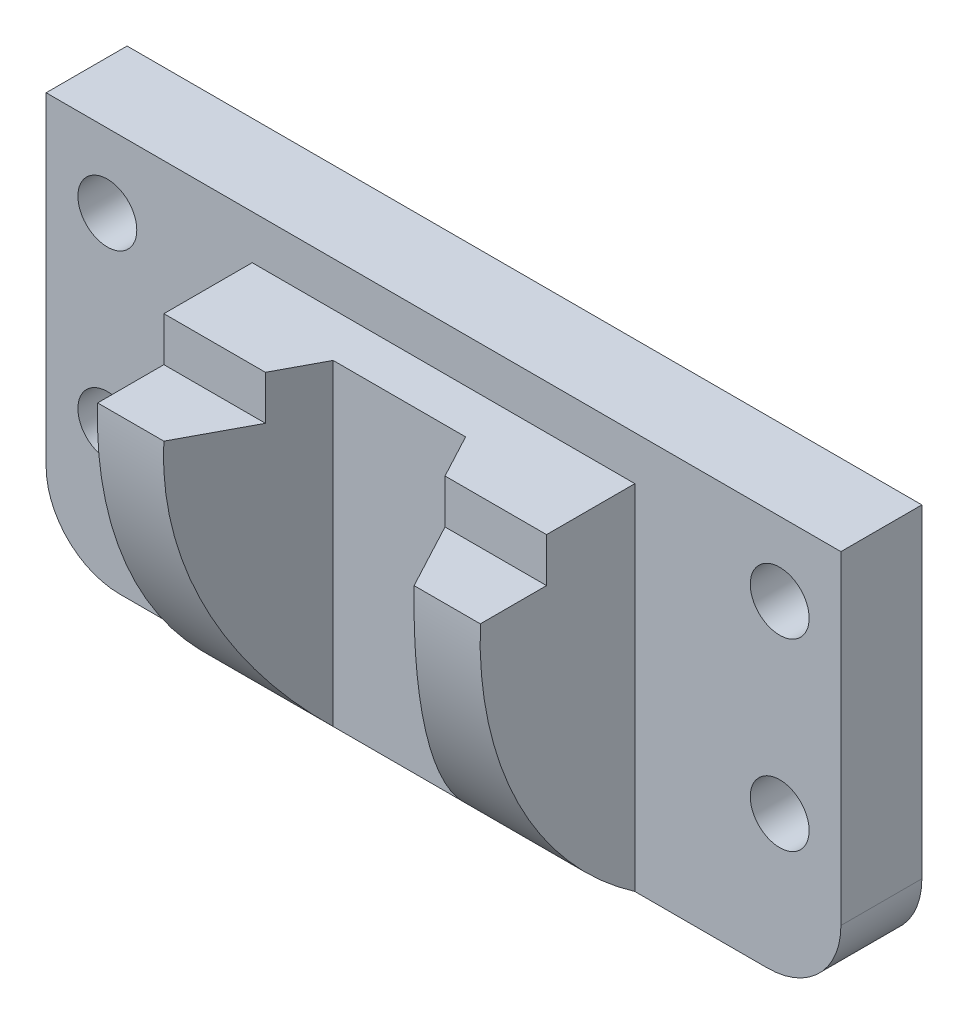
ISO-10303-21;
HEADER;
FILE_DESCRIPTION(('STEP AP214'),'2;1');
FILE_NAME('part.step','',(''),(''),'','','');
FILE_SCHEMA(('AUTOMOTIVE_DESIGN { 1 0 10303 214 1 1 1 1 }'));
ENDSEC;
DATA;
#1=APPLICATION_CONTEXT('core data for automotive mechanical design processes');
#2=APPLICATION_PROTOCOL_DEFINITION('international standard','automotive_design',2000,#1);
#3=PRODUCT_CONTEXT('',#1,'mechanical');
#4=PRODUCT('Part','Part','',(#3));
#5=PRODUCT_RELATED_PRODUCT_CATEGORY('part','',(#4));
#6=PRODUCT_DEFINITION_FORMATION('','',#4);
#7=PRODUCT_DEFINITION_CONTEXT('part definition',#1,'design');
#8=PRODUCT_DEFINITION('design','',#6,#7);
#9=PRODUCT_DEFINITION_SHAPE('','',#8);
#10=(LENGTH_UNIT() NAMED_UNIT(*) SI_UNIT(.MILLI.,.METRE.));
#11=(NAMED_UNIT(*) PLANE_ANGLE_UNIT() SI_UNIT($,.RADIAN.));
#12=(NAMED_UNIT(*) SI_UNIT($,.STERADIAN.) SOLID_ANGLE_UNIT());
#13=UNCERTAINTY_MEASURE_WITH_UNIT(LENGTH_MEASURE(1.E-05),#10,'distance_accuracy_value','');
#14=(GEOMETRIC_REPRESENTATION_CONTEXT(3) GLOBAL_UNCERTAINTY_ASSIGNED_CONTEXT((#13)) GLOBAL_UNIT_ASSIGNED_CONTEXT((#10,
#11,#12)) REPRESENTATION_CONTEXT('',''));
#15=CARTESIAN_POINT('',(0.,0.,0.));
#16=DIRECTION('',(0.,0.,1.));
#17=DIRECTION('',(1.,0.,0.));
#18=AXIS2_PLACEMENT_3D('',#15,#16,#17);
#19=CARTESIAN_POINT('',(26.,21.,23.));
#20=DIRECTION('',(0.,0.,-1.));
#21=DIRECTION('',(0.,1.,0.));
#22=AXIS2_PLACEMENT_3D('',#19,#20,#21);
#23=PLANE('',#22);
#24=DIRECTION('',(-1.,0.,0.));
#25=VECTOR('',#24,1.);
#26=CARTESIAN_POINT('',(26.,21.,23.));
#27=LINE('',#26,#25);
#28=CARTESIAN_POINT('',(26.,21.,23.));
#29=VERTEX_POINT('',#28);
#30=CARTESIAN_POINT('',(12.2,21.,23.));
#31=VERTEX_POINT('',#30);
#32=EDGE_CURVE('E242',#29,#31,#27,.T.);
#33=ORIENTED_EDGE('',*,*,#32,.T.);
#34=DIRECTION('',(0.,-1.,0.));
#35=VECTOR('',#34,1.);
#36=CARTESIAN_POINT('',(12.2,21.,23.));
#37=LINE('',#36,#35);
#38=CARTESIAN_POINT('',(12.2,15.,23.));
#39=VERTEX_POINT('',#38);
#40=EDGE_CURVE('E283',#31,#39,#37,.T.);
#41=ORIENTED_EDGE('',*,*,#40,.T.);
#42=DIRECTION('',(-1.,0.,0.));
#43=VECTOR('',#42,1.);
#44=CARTESIAN_POINT('',(26.,15.,23.));
#45=LINE('',#44,#43);
#46=CARTESIAN_POINT('',(26.,15.,23.));
#47=VERTEX_POINT('',#46);
#48=EDGE_CURVE('E246',#47,#39,#45,.T.);
#49=ORIENTED_EDGE('',*,*,#48,.F.);
#50=DIRECTION('',(0.,-1.,0.));
#51=VECTOR('',#50,1.);
#52=CARTESIAN_POINT('',(26.,21.,23.));
#53=LINE('',#52,#51);
#54=EDGE_CURVE('E274',#29,#47,#53,.T.);
#55=ORIENTED_EDGE('',*,*,#54,.F.);
#56=EDGE_LOOP('',(#33,#41,#49,#55));
#57=FACE_BOUND('',#56,.T.);
#58=ADVANCED_FACE('F39',(#57),#23,.F.);
#59=CARTESIAN_POINT('',(26.,15.,23.));
#60=DIRECTION('',(0.,-1.,0.));
#61=DIRECTION('',(0.,0.,-1.));
#62=AXIS2_PLACEMENT_3D('',#59,#60,#61);
#63=PLANE('',#62);
#64=ORIENTED_EDGE('',*,*,#48,.T.);
#65=DIRECTION('',(0.470588235294118,0.,0.882352941176471));
#66=VECTOR('',#65,1.);
#67=CARTESIAN_POINT('',(15.2560553633218,15.,28.7301038062284));
#68=LINE('',#67,#66);
#69=CARTESIAN_POINT('',(17.,15.,32.));
#70=VERTEX_POINT('',#69);
#71=EDGE_CURVE('E286',#39,#70,#68,.T.);
#72=ORIENTED_EDGE('',*,*,#71,.T.);
#73=DIRECTION('',(-1.,0.,0.));
#74=VECTOR('',#73,1.);
#75=CARTESIAN_POINT('',(26.,15.,32.));
#76=LINE('',#75,#74);
#77=CARTESIAN_POINT('',(26.,15.,32.));
#78=VERTEX_POINT('',#77);
#79=EDGE_CURVE('E253',#78,#70,#76,.T.);
#80=ORIENTED_EDGE('',*,*,#79,.F.);
#81=DIRECTION('',(0.,0.,1.));
#82=VECTOR('',#81,1.);
#83=CARTESIAN_POINT('',(26.,15.,23.));
#84=LINE('',#83,#82);
#85=EDGE_CURVE('E272',#47,#78,#84,.T.);
#86=ORIENTED_EDGE('',*,*,#85,.F.);
#87=EDGE_LOOP('',(#64,#72,#80,#86));
#88=FACE_BOUND('',#87,.T.);
#89=ADVANCED_FACE('F355',(#88),#63,.F.);
#90=CARTESIAN_POINT('',(-44.,-17.,11.));
#91=DIRECTION('',(0.,0.,1.));
#92=DIRECTION('',(1.,0.,0.));
#93=AXIS2_PLACEMENT_3D('',#90,#91,#92);
#94=PLANE('',#93);
#95=CARTESIAN_POINT('',(45.6822643330834,-8.,11.));
#96=DIRECTION('',(0.,0.,1.));
#97=DIRECTION('',(-1.,0.,0.));
#98=AXIS2_PLACEMENT_3D('',#95,#96,#97);
#99=CIRCLE('',#98,4.00000000000001);
#100=CARTESIAN_POINT('',(41.6822643330834,-8.,11.));
#101=VERTEX_POINT('',#100);
#102=EDGE_CURVE('E226',#101,#101,#99,.T.);
#103=ORIENTED_EDGE('',*,*,#102,.F.);
#104=EDGE_LOOP('',(#103));
#105=FACE_BOUND('',#104,.T.);
#106=CARTESIAN_POINT('',(-45.6822643330834,17.,11.));
#107=DIRECTION('',(0.,0.,1.));
#108=DIRECTION('',(1.,0.,0.));
#109=AXIS2_PLACEMENT_3D('',#106,#107,#108);
#110=CIRCLE('',#109,4.00000000000001);
#111=CARTESIAN_POINT('',(-41.6822643330834,17.,11.));
#112=VERTEX_POINT('',#111);
#113=EDGE_CURVE('E201',#112,#112,#110,.T.);
#114=ORIENTED_EDGE('',*,*,#113,.F.);
#115=EDGE_LOOP('',(#114));
#116=FACE_BOUND('',#115,.T.);
#117=CARTESIAN_POINT('',(-45.6822643330834,-8.00000000000001,11.));
#118=DIRECTION('',(0.,0.,1.));
#119=DIRECTION('',(1.,0.,0.));
#120=AXIS2_PLACEMENT_3D('',#117,#118,#119);
#121=CIRCLE('',#120,4.00000000000001);
#122=CARTESIAN_POINT('',(-41.6822643330834,-8.00000000000001,11.));
#123=VERTEX_POINT('',#122);
#124=EDGE_CURVE('E219',#123,#123,#121,.T.);
#125=ORIENTED_EDGE('',*,*,#124,.F.);
#126=EDGE_LOOP('',(#125));
#127=FACE_BOUND('',#126,.T.);
#128=CARTESIAN_POINT('',(45.6822643330834,17.,11.));
#129=DIRECTION('',(0.,0.,1.));
#130=DIRECTION('',(-1.,0.,0.));
#131=AXIS2_PLACEMENT_3D('',#128,#129,#130);
#132=CIRCLE('',#131,4.);
#133=CARTESIAN_POINT('',(41.6822643330834,17.,11.));
#134=VERTEX_POINT('',#133);
#135=EDGE_CURVE('E231',#134,#134,#132,.T.);
#136=ORIENTED_EDGE('',*,*,#135,.F.);
#137=EDGE_LOOP('',(#136));
#138=FACE_BOUND('',#137,.T.);
#139=DIRECTION('',(1.,0.,0.));
#140=VECTOR('',#139,1.);
#141=CARTESIAN_POINT('',(-43.9999999999999,-27.,11.));
#142=LINE('',#141,#140);
#143=CARTESIAN_POINT('',(-43.9999999999999,-27.,11.));
#144=VERTEX_POINT('',#143);
#145=CARTESIAN_POINT('',(-26.,-27.,11.));
#146=VERTEX_POINT('',#145);
#147=EDGE_CURVE('E207',#144,#146,#142,.T.);
#148=ORIENTED_EDGE('',*,*,#147,.T.);
#149=DIRECTION('',(0.,1.,0.));
#150=VECTOR('',#149,1.);
#151=CARTESIAN_POINT('',(-26.,21.,11.));
#152=LINE('',#151,#150);
#153=CARTESIAN_POINT('',(-26.,21.,11.));
#154=VERTEX_POINT('',#153);
#155=EDGE_CURVE('E267',#146,#154,#152,.T.);
#156=ORIENTED_EDGE('',*,*,#155,.T.);
#157=DIRECTION('',(-1.,0.,0.));
#158=VECTOR('',#157,1.);
#159=CARTESIAN_POINT('',(26.,21.,11.));
#160=LINE('',#159,#158);
#161=CARTESIAN_POINT('',(26.,21.,11.));
#162=VERTEX_POINT('',#161);
#163=EDGE_CURVE('E236',#162,#154,#160,.T.);
#164=ORIENTED_EDGE('',*,*,#163,.F.);
#165=DIRECTION('',(0.,1.,0.));
#166=VECTOR('',#165,1.);
#167=CARTESIAN_POINT('',(26.,21.,11.));
#168=LINE('',#167,#166);
#169=CARTESIAN_POINT('',(26.,-27.,11.));
#170=VERTEX_POINT('',#169);
#171=EDGE_CURVE('E65',#170,#162,#168,.T.);
#172=ORIENTED_EDGE('',*,*,#171,.F.);
#173=CARTESIAN_POINT('',(43.9999999999999,-27.,11.));
#174=VERTEX_POINT('',#173);
#175=EDGE_CURVE('E215',#170,#174,#142,.T.);
#176=ORIENTED_EDGE('',*,*,#175,.T.);
#177=CARTESIAN_POINT('',(44.,-17.,11.));
#178=DIRECTION('',(0.,0.,1.));
#179=DIRECTION('',(1.,0.,0.));
#180=AXIS2_PLACEMENT_3D('',#177,#178,#179);
#181=CIRCLE('',#180,10.);
#182=CARTESIAN_POINT('',(54.,-16.9999999999999,11.));
#183=VERTEX_POINT('',#182);
#184=EDGE_CURVE('E210',#174,#183,#181,.T.);
#185=ORIENTED_EDGE('',*,*,#184,.T.);
#186=DIRECTION('',(0.,1.,0.));
#187=VECTOR('',#186,1.);
#188=CARTESIAN_POINT('',(54.,27.,11.));
#189=LINE('',#188,#187);
#190=CARTESIAN_POINT('',(54.,27.,11.));
#191=VERTEX_POINT('',#190);
#192=EDGE_CURVE('E202',#183,#191,#189,.T.);
#193=ORIENTED_EDGE('',*,*,#192,.T.);
#194=DIRECTION('',(-1.,0.,0.));
#195=VECTOR('',#194,1.);
#196=CARTESIAN_POINT('',(-54.,27.,11.));
#197=LINE('',#196,#195);
#198=CARTESIAN_POINT('',(-54.,27.,11.));
#199=VERTEX_POINT('',#198);
#200=EDGE_CURVE('E187',#191,#199,#197,.T.);
#201=ORIENTED_EDGE('',*,*,#200,.T.);
#202=DIRECTION('',(0.,-1.,0.));
#203=VECTOR('',#202,1.);
#204=CARTESIAN_POINT('',(-54.,27.,11.));
#205=LINE('',#204,#203);
#206=CARTESIAN_POINT('',(-54.,-16.9999999999999,11.));
#207=VERTEX_POINT('',#206);
#208=EDGE_CURVE('E194',#199,#207,#205,.T.);
#209=ORIENTED_EDGE('',*,*,#208,.T.);
#210=CARTESIAN_POINT('',(-44.,-17.,11.));
#211=DIRECTION('',(0.,0.,1.));
#212=DIRECTION('',(1.,0.,0.));
#213=AXIS2_PLACEMENT_3D('',#210,#211,#212);
#214=CIRCLE('',#213,10.);
#215=EDGE_CURVE('E213',#207,#144,#214,.T.);
#216=ORIENTED_EDGE('',*,*,#215,.T.);
#217=EDGE_LOOP('',(#148,#156,#164,#172,#176,#185,#193,#201,#209,#216));
#218=FACE_BOUND('',#217,.T.);
#219=ADVANCED_FACE('F321',(#105,#116,#127,#138,#218),#94,.T.);
#220=CARTESIAN_POINT('',(-44.,-17.,0.));
#221=DIRECTION('',(0.,0.,1.));
#222=DIRECTION('',(1.,0.,0.));
#223=AXIS2_PLACEMENT_3D('',#220,#221,#222);
#224=PLANE('',#223);
#225=DIRECTION('',(0.,-1.,0.));
#226=VECTOR('',#225,1.);
#227=CARTESIAN_POINT('',(-54.,27.,0.));
#228=LINE('',#227,#226);
#229=CARTESIAN_POINT('',(-54.,27.,0.));
#230=VERTEX_POINT('',#229);
#231=CARTESIAN_POINT('',(-54.,-16.9999999999999,0.));
#232=VERTEX_POINT('',#231);
#233=EDGE_CURVE('E199',#230,#232,#228,.T.);
#234=ORIENTED_EDGE('',*,*,#233,.F.);
#235=DIRECTION('',(-1.,0.,0.));
#236=VECTOR('',#235,1.);
#237=CARTESIAN_POINT('',(-54.,27.,0.));
#238=LINE('',#237,#236);
#239=CARTESIAN_POINT('',(54.,27.,0.));
#240=VERTEX_POINT('',#239);
#241=EDGE_CURVE('E188',#240,#230,#238,.T.);
#242=ORIENTED_EDGE('',*,*,#241,.F.);
#243=DIRECTION('',(0.,1.,0.));
#244=VECTOR('',#243,1.);
#245=CARTESIAN_POINT('',(54.,27.,0.));
#246=LINE('',#245,#244);
#247=CARTESIAN_POINT('',(54.,-16.9999999999999,0.));
#248=VERTEX_POINT('',#247);
#249=EDGE_CURVE('E191',#248,#240,#246,.T.);
#250=ORIENTED_EDGE('',*,*,#249,.F.);
#251=CARTESIAN_POINT('',(44.,-17.,0.));
#252=DIRECTION('',(0.,0.,1.));
#253=DIRECTION('',(1.,0.,0.));
#254=AXIS2_PLACEMENT_3D('',#251,#252,#253);
#255=CIRCLE('',#254,10.);
#256=CARTESIAN_POINT('',(43.9999999999999,-27.,0.));
#257=VERTEX_POINT('',#256);
#258=EDGE_CURVE('E193',#257,#248,#255,.T.);
#259=ORIENTED_EDGE('',*,*,#258,.F.);
#260=DIRECTION('',(1.,0.,0.));
#261=VECTOR('',#260,1.);
#262=CARTESIAN_POINT('',(-43.9999999999999,-27.,0.));
#263=LINE('',#262,#261);
#264=CARTESIAN_POINT('',(-43.9999999999999,-27.,0.));
#265=VERTEX_POINT('',#264);
#266=EDGE_CURVE('E198',#265,#257,#263,.T.);
#267=ORIENTED_EDGE('',*,*,#266,.F.);
#268=CARTESIAN_POINT('',(-44.,-17.,0.));
#269=DIRECTION('',(0.,0.,1.));
#270=DIRECTION('',(1.,0.,0.));
#271=AXIS2_PLACEMENT_3D('',#268,#269,#270);
#272=CIRCLE('',#271,10.);
#273=EDGE_CURVE('E196',#232,#265,#272,.T.);
#274=ORIENTED_EDGE('',*,*,#273,.F.);
#275=EDGE_LOOP('',(#234,#242,#250,#259,#267,#274));
#276=FACE_BOUND('',#275,.T.);
#277=CARTESIAN_POINT('',(-45.6822643330834,17.,0.));
#278=DIRECTION('',(0.,0.,1.));
#279=DIRECTION('',(1.,0.,0.));
#280=AXIS2_PLACEMENT_3D('',#277,#278,#279);
#281=CIRCLE('',#280,4.00000000000001);
#282=CARTESIAN_POINT('',(-41.6822643330834,17.,0.));
#283=VERTEX_POINT('',#282);
#284=EDGE_CURVE('E220',#283,#283,#281,.T.);
#285=ORIENTED_EDGE('',*,*,#284,.T.);
#286=EDGE_LOOP('',(#285));
#287=FACE_BOUND('',#286,.T.);
#288=CARTESIAN_POINT('',(-45.6822643330834,-8.00000000000001,0.));
#289=DIRECTION('',(0.,0.,1.));
#290=DIRECTION('',(1.,0.,0.));
#291=AXIS2_PLACEMENT_3D('',#288,#289,#290);
#292=CIRCLE('',#291,4.00000000000001);
#293=CARTESIAN_POINT('',(-41.6822643330834,-8.00000000000001,0.));
#294=VERTEX_POINT('',#293);
#295=EDGE_CURVE('E224',#294,#294,#292,.T.);
#296=ORIENTED_EDGE('',*,*,#295,.T.);
#297=EDGE_LOOP('',(#296));
#298=FACE_BOUND('',#297,.T.);
#299=CARTESIAN_POINT('',(45.6822643330834,-8.,0.));
#300=DIRECTION('',(0.,0.,1.));
#301=DIRECTION('',(-1.,0.,0.));
#302=AXIS2_PLACEMENT_3D('',#299,#300,#301);
#303=CIRCLE('',#302,4.00000000000001);
#304=CARTESIAN_POINT('',(41.6822643330834,-8.,0.));
#305=VERTEX_POINT('',#304);
#306=EDGE_CURVE('E228',#305,#305,#303,.T.);
#307=ORIENTED_EDGE('',*,*,#306,.T.);
#308=EDGE_LOOP('',(#307));
#309=FACE_BOUND('',#308,.T.);
#310=CARTESIAN_POINT('',(45.6822643330834,17.,0.));
#311=DIRECTION('',(0.,0.,1.));
#312=DIRECTION('',(-1.,0.,0.));
#313=AXIS2_PLACEMENT_3D('',#310,#311,#312);
#314=CIRCLE('',#313,4.);
#315=CARTESIAN_POINT('',(41.6822643330834,17.,0.));
#316=VERTEX_POINT('',#315);
#317=EDGE_CURVE('E232',#316,#316,#314,.T.);
#318=ORIENTED_EDGE('',*,*,#317,.T.);
#319=EDGE_LOOP('',(#318));
#320=FACE_BOUND('',#319,.T.);
#321=ADVANCED_FACE('F332',(#276,#287,#298,#309,#320),#224,.F.);
#322=CARTESIAN_POINT('',(-54.,27.,11.));
#323=DIRECTION('',(1.,0.,0.));
#324=DIRECTION('',(0.,1.,0.));
#325=AXIS2_PLACEMENT_3D('',#322,#323,#324);
#326=PLANE('',#325);
#327=ORIENTED_EDGE('',*,*,#233,.T.);
#328=DIRECTION('',(0.,0.,-1.));
#329=VECTOR('',#328,1.);
#330=CARTESIAN_POINT('',(-54.,-16.9999999999999,11.));
#331=LINE('',#330,#329);
#332=EDGE_CURVE('E158',#207,#232,#331,.T.);
#333=ORIENTED_EDGE('',*,*,#332,.F.);
#334=ORIENTED_EDGE('',*,*,#208,.F.);
#335=DIRECTION('',(0.,0.,-1.));
#336=VECTOR('',#335,1.);
#337=CARTESIAN_POINT('',(-54.,27.,11.));
#338=LINE('',#337,#336);
#339=EDGE_CURVE('E183',#199,#230,#338,.T.);
#340=ORIENTED_EDGE('',*,*,#339,.T.);
#341=EDGE_LOOP('',(#327,#333,#334,#340));
#342=FACE_BOUND('',#341,.T.);
#343=ADVANCED_FACE('F41',(#342),#326,.F.);
#344=CARTESIAN_POINT('',(-44.,-17.,11.));
#345=DIRECTION('',(0.,0.,-1.));
#346=DIRECTION('',(-1.,0.,0.));
#347=AXIS2_PLACEMENT_3D('',#344,#345,#346);
#348=CYLINDRICAL_SURFACE('',#347,10.);
#349=ORIENTED_EDGE('',*,*,#273,.T.);
#350=DIRECTION('',(0.,0.,-1.));
#351=VECTOR('',#350,1.);
#352=CARTESIAN_POINT('',(-43.9999999999999,-27.,11.));
#353=LINE('',#352,#351);
#354=EDGE_CURVE('E172',#144,#265,#353,.T.);
#355=ORIENTED_EDGE('',*,*,#354,.F.);
#356=ORIENTED_EDGE('',*,*,#215,.F.);
#357=ORIENTED_EDGE('',*,*,#332,.T.);
#358=EDGE_LOOP('',(#349,#355,#356,#357));
#359=FACE_BOUND('',#358,.T.);
#360=ADVANCED_FACE('F326',(#359),#348,.T.);
#361=CARTESIAN_POINT('',(-43.9999999999999,-27.,11.));
#362=DIRECTION('',(0.,1.,0.));
#363=DIRECTION('',(0.,0.,1.));
#364=AXIS2_PLACEMENT_3D('',#361,#362,#363);
#365=PLANE('',#364);
#366=ORIENTED_EDGE('',*,*,#266,.T.);
#367=DIRECTION('',(0.,0.,-1.));
#368=VECTOR('',#367,1.);
#369=CARTESIAN_POINT('',(43.9999999999999,-27.,11.));
#370=LINE('',#369,#368);
#371=EDGE_CURVE('E179',#174,#257,#370,.T.);
#372=ORIENTED_EDGE('',*,*,#371,.F.);
#373=ORIENTED_EDGE('',*,*,#175,.F.);
#374=DIRECTION('',(-1.,0.,0.));
#375=VECTOR('',#374,1.);
#376=CARTESIAN_POINT('',(26.,-27.,11.));
#377=LINE('',#376,#375);
#378=EDGE_CURVE('E255',#170,#146,#377,.T.);
#379=ORIENTED_EDGE('',*,*,#378,.T.);
#380=ORIENTED_EDGE('',*,*,#147,.F.);
#381=ORIENTED_EDGE('',*,*,#354,.T.);
#382=EDGE_LOOP('',(#366,#372,#373,#379,#380,#381));
#383=FACE_BOUND('',#382,.T.);
#384=ADVANCED_FACE('F317',(#383),#365,.F.);
#385=CARTESIAN_POINT('',(44.,-17.,11.));
#386=DIRECTION('',(0.,0.,-1.));
#387=DIRECTION('',(-1.,0.,0.));
#388=AXIS2_PLACEMENT_3D('',#385,#386,#387);
#389=CYLINDRICAL_SURFACE('',#388,10.);
#390=ORIENTED_EDGE('',*,*,#258,.T.);
#391=DIRECTION('',(0.,0.,-1.));
#392=VECTOR('',#391,1.);
#393=CARTESIAN_POINT('',(54.,-16.9999999999999,11.));
#394=LINE('',#393,#392);
#395=EDGE_CURVE('E178',#183,#248,#394,.T.);
#396=ORIENTED_EDGE('',*,*,#395,.F.);
#397=ORIENTED_EDGE('',*,*,#184,.F.);
#398=ORIENTED_EDGE('',*,*,#371,.T.);
#399=EDGE_LOOP('',(#390,#396,#397,#398));
#400=FACE_BOUND('',#399,.T.);
#401=ADVANCED_FACE('F340',(#400),#389,.T.);
#402=CARTESIAN_POINT('',(54.,27.,11.));
#403=DIRECTION('',(-1.,0.,0.));
#404=DIRECTION('',(0.,-1.,0.));
#405=AXIS2_PLACEMENT_3D('',#402,#403,#404);
#406=PLANE('',#405);
#407=ORIENTED_EDGE('',*,*,#249,.T.);
#408=DIRECTION('',(0.,0.,-1.));
#409=VECTOR('',#408,1.);
#410=CARTESIAN_POINT('',(54.,27.,11.));
#411=LINE('',#410,#409);
#412=EDGE_CURVE('E185',#191,#240,#411,.T.);
#413=ORIENTED_EDGE('',*,*,#412,.F.);
#414=ORIENTED_EDGE('',*,*,#192,.F.);
#415=ORIENTED_EDGE('',*,*,#395,.T.);
#416=EDGE_LOOP('',(#407,#413,#414,#415));
#417=FACE_BOUND('',#416,.T.);
#418=ADVANCED_FACE('F344',(#417),#406,.F.);
#419=CARTESIAN_POINT('',(-54.,27.,11.));
#420=DIRECTION('',(0.,-1.,0.));
#421=DIRECTION('',(0.,0.,-1.));
#422=AXIS2_PLACEMENT_3D('',#419,#420,#421);
#423=PLANE('',#422);
#424=ORIENTED_EDGE('',*,*,#241,.T.);
#425=ORIENTED_EDGE('',*,*,#339,.F.);
#426=ORIENTED_EDGE('',*,*,#200,.F.);
#427=ORIENTED_EDGE('',*,*,#412,.T.);
#428=EDGE_LOOP('',(#424,#425,#426,#427));
#429=FACE_BOUND('',#428,.T.);
#430=ADVANCED_FACE('F392',(#429),#423,.F.);
#431=CARTESIAN_POINT('',(-45.6822643330834,17.,11.));
#432=DIRECTION('',(0.,0.,-1.));
#433=DIRECTION('',(-1.,0.,0.));
#434=AXIS2_PLACEMENT_3D('',#431,#432,#433);
#435=CYLINDRICAL_SURFACE('',#434,4.00000000000001);
#436=ORIENTED_EDGE('',*,*,#113,.T.);
#437=EDGE_LOOP('',(#436));
#438=FACE_BOUND('',#437,.T.);
#439=ORIENTED_EDGE('',*,*,#284,.F.);
#440=EDGE_LOOP('',(#439));
#441=FACE_BOUND('',#440,.T.);
#442=ADVANCED_FACE('F386',(#438,#441),#435,.F.);
#443=CARTESIAN_POINT('',(-45.6822643330834,-8.00000000000001,11.));
#444=DIRECTION('',(0.,0.,-1.));
#445=DIRECTION('',(-1.,0.,0.));
#446=AXIS2_PLACEMENT_3D('',#443,#444,#445);
#447=CYLINDRICAL_SURFACE('',#446,4.00000000000001);
#448=ORIENTED_EDGE('',*,*,#124,.T.);
#449=EDGE_LOOP('',(#448));
#450=FACE_BOUND('',#449,.T.);
#451=ORIENTED_EDGE('',*,*,#295,.F.);
#452=EDGE_LOOP('',(#451));
#453=FACE_BOUND('',#452,.T.);
#454=ADVANCED_FACE('F384',(#450,#453),#447,.F.);
#455=CARTESIAN_POINT('',(45.6822643330834,-8.,11.));
#456=DIRECTION('',(0.,0.,-1.));
#457=DIRECTION('',(-1.,0.,0.));
#458=AXIS2_PLACEMENT_3D('',#455,#456,#457);
#459=CYLINDRICAL_SURFACE('',#458,4.00000000000001);
#460=ORIENTED_EDGE('',*,*,#102,.T.);
#461=EDGE_LOOP('',(#460));
#462=FACE_BOUND('',#461,.T.);
#463=ORIENTED_EDGE('',*,*,#306,.F.);
#464=EDGE_LOOP('',(#463));
#465=FACE_BOUND('',#464,.T.);
#466=ADVANCED_FACE('F377',(#462,#465),#459,.F.);
#467=CARTESIAN_POINT('',(45.6822643330834,17.,11.));
#468=DIRECTION('',(0.,0.,-1.));
#469=DIRECTION('',(-1.,0.,0.));
#470=AXIS2_PLACEMENT_3D('',#467,#468,#469);
#471=CYLINDRICAL_SURFACE('',#470,4.);
#472=ORIENTED_EDGE('',*,*,#135,.T.);
#473=EDGE_LOOP('',(#472));
#474=FACE_BOUND('',#473,.T.);
#475=ORIENTED_EDGE('',*,*,#317,.F.);
#476=EDGE_LOOP('',(#475));
#477=FACE_BOUND('',#476,.T.);
#478=ADVANCED_FACE('F374',(#474,#477),#471,.F.);
#479=CARTESIAN_POINT('',(26.,21.,11.));
#480=DIRECTION('',(0.,-1.,0.));
#481=DIRECTION('',(0.,0.,-1.));
#482=AXIS2_PLACEMENT_3D('',#479,#480,#481);
#483=PLANE('',#482);
#484=DIRECTION('',(1.,0.,0.));
#485=VECTOR('',#484,1.);
#486=CARTESIAN_POINT('',(26.,21.,17.));
#487=LINE('',#486,#485);
#488=CARTESIAN_POINT('',(-9.,21.,17.));
#489=VERTEX_POINT('',#488);
#490=CARTESIAN_POINT('',(9.,21.,17.));
#491=VERTEX_POINT('',#490);
#492=EDGE_CURVE('E164',#489,#491,#487,.T.);
#493=ORIENTED_EDGE('',*,*,#492,.T.);
#494=DIRECTION('',(0.470588235294118,0.,0.882352941176471));
#495=VECTOR('',#494,1.);
#496=CARTESIAN_POINT('',(10.2733564013841,21.,19.3875432525952));
#497=LINE('',#496,#495);
#498=EDGE_CURVE('E281',#491,#31,#497,.T.);
#499=ORIENTED_EDGE('',*,*,#498,.T.);
#500=ORIENTED_EDGE('',*,*,#32,.F.);
#501=DIRECTION('',(0.,0.,1.));
#502=VECTOR('',#501,1.);
#503=CARTESIAN_POINT('',(26.,21.,11.));
#504=LINE('',#503,#502);
#505=EDGE_CURVE('E280',#162,#29,#504,.T.);
#506=ORIENTED_EDGE('',*,*,#505,.F.);
#507=ORIENTED_EDGE('',*,*,#163,.T.);
#508=DIRECTION('',(0.,0.,1.));
#509=VECTOR('',#508,1.);
#510=CARTESIAN_POINT('',(-26.,21.,11.));
#511=LINE('',#510,#509);
#512=CARTESIAN_POINT('',(-26.,21.,23.));
#513=VERTEX_POINT('',#512);
#514=EDGE_CURVE('E266',#154,#513,#511,.T.);
#515=ORIENTED_EDGE('',*,*,#514,.T.);
#516=CARTESIAN_POINT('',(-12.2,21.,23.));
#517=VERTEX_POINT('',#516);
#518=EDGE_CURVE('E249',#517,#513,#27,.T.);
#519=ORIENTED_EDGE('',*,*,#518,.F.);
#520=DIRECTION('',(0.470588235294118,0.,-0.882352941176471));
#521=VECTOR('',#520,1.);
#522=CARTESIAN_POINT('',(1.24221453287198,21.,-2.20415224913495));
#523=LINE('',#522,#521);
#524=EDGE_CURVE('E287',#517,#489,#523,.T.);
#525=ORIENTED_EDGE('',*,*,#524,.T.);
#526=EDGE_LOOP('',(#493,#499,#500,#506,#507,#515,#519,#525));
#527=FACE_BOUND('',#526,.T.);
#528=ADVANCED_FACE('F297',(#527),#483,.F.);
#529=CARTESIAN_POINT('',(-12.2,15.,23.));
#530=VERTEX_POINT('',#529);
#531=CARTESIAN_POINT('',(-26.,15.,23.));
#532=VERTEX_POINT('',#531);
#533=EDGE_CURVE('E247',#530,#532,#45,.T.);
#534=ORIENTED_EDGE('',*,*,#533,.F.);
#535=DIRECTION('',(0.,1.,0.));
#536=VECTOR('',#535,1.);
#537=CARTESIAN_POINT('',(-12.2,21.,23.));
#538=LINE('',#537,#536);
#539=EDGE_CURVE('E295',#530,#517,#538,.T.);
#540=ORIENTED_EDGE('',*,*,#539,.T.);
#541=ORIENTED_EDGE('',*,*,#518,.T.);
#542=DIRECTION('',(0.,-1.,0.));
#543=VECTOR('',#542,1.);
#544=CARTESIAN_POINT('',(-26.,21.,23.));
#545=LINE('',#544,#543);
#546=EDGE_CURVE('E263',#513,#532,#545,.T.);
#547=ORIENTED_EDGE('',*,*,#546,.T.);
#548=EDGE_LOOP('',(#534,#540,#541,#547));
#549=FACE_BOUND('',#548,.T.);
#550=ADVANCED_FACE('F305',(#549),#23,.F.);
#551=CARTESIAN_POINT('',(-17.,15.,32.));
#552=VERTEX_POINT('',#551);
#553=CARTESIAN_POINT('',(-26.,15.,32.));
#554=VERTEX_POINT('',#553);
#555=EDGE_CURVE('E251',#552,#554,#76,.T.);
#556=ORIENTED_EDGE('',*,*,#555,.F.);
#557=DIRECTION('',(0.470588235294118,0.,-0.882352941176471));
#558=VECTOR('',#557,1.);
#559=CARTESIAN_POINT('',(-3.74048442906574,15.,7.13840830449827));
#560=LINE('',#559,#558);
#561=EDGE_CURVE('E53',#552,#530,#560,.T.);
#562=ORIENTED_EDGE('',*,*,#561,.T.);
#563=ORIENTED_EDGE('',*,*,#533,.T.);
#564=DIRECTION('',(0.,0.,1.));
#565=VECTOR('',#564,1.);
#566=CARTESIAN_POINT('',(-26.,15.,23.));
#567=LINE('',#566,#565);
#568=EDGE_CURVE('E257',#532,#554,#567,.T.);
#569=ORIENTED_EDGE('',*,*,#568,.T.);
#570=EDGE_LOOP('',(#556,#562,#563,#569));
#571=FACE_BOUND('',#570,.T.);
#572=ADVANCED_FACE('F307',(#571),#63,.F.);
#573=CARTESIAN_POINT('',(26.,13.2340843296477,-16.9681686592954));
#574=DIRECTION('',(-1.,0.,0.));
#575=DIRECTION('',(0.,0.,1.));
#576=AXIS2_PLACEMENT_3D('',#573,#574,#575);
#577=CYLINDRICAL_SURFACE('',#576,49.);
#578=ORIENTED_EDGE('',*,*,#79,.T.);
#579=CARTESIAN_POINT('',(-9.11635661829091,13.2340843296477,-16.9681686592954));
#580=DIRECTION('',(0.88235294117647,0.,-0.470588235294118));
#581=DIRECTION('',(-0.470588235294118,0.,-0.882352941176471));
#582=AXIS2_PLACEMENT_3D('',#579,#580,#581);
#583=ELLIPSE('',#582,55.5333333333333,49.);
#584=CARTESIAN_POINT('',(9.,-22.0811180332676,17.));
#585=VERTEX_POINT('',#584);
#586=EDGE_CURVE('E11',#70,#585,#583,.T.);
#587=ORIENTED_EDGE('',*,*,#586,.T.);
#588=DIRECTION('',(-1.,0.,0.));
#589=VECTOR('',#588,1.);
#590=CARTESIAN_POINT('',(26.,-22.0811180332676,17.));
#591=LINE('',#590,#589);
#592=CARTESIAN_POINT('',(-9.,-22.0811180332676,17.));
#593=VERTEX_POINT('',#592);
#594=EDGE_CURVE('E50',#585,#593,#591,.T.);
#595=ORIENTED_EDGE('',*,*,#594,.T.);
#596=CARTESIAN_POINT('',(9.11635661829091,13.2340843296477,-16.9681686592954));
#597=DIRECTION('',(-0.882352941176471,0.,-0.470588235294118));
#598=DIRECTION('',(-0.470588235294118,0.,0.882352941176471));
#599=AXIS2_PLACEMENT_3D('',#596,#597,#598);
#600=ELLIPSE('',#599,55.5333333333333,49.);
#601=EDGE_CURVE('E147',#593,#552,#600,.T.);
#602=ORIENTED_EDGE('',*,*,#601,.T.);
#603=ORIENTED_EDGE('',*,*,#555,.T.);
#604=CARTESIAN_POINT('',(-26.,13.2340843296477,-16.9681686592954));
#605=DIRECTION('',(1.,0.,0.));
#606=DIRECTION('',(0.,0.,-1.));
#607=AXIS2_PLACEMENT_3D('',#604,#605,#606);
#608=CIRCLE('',#607,49.);
#609=EDGE_CURVE('E256',#554,#146,#608,.T.);
#610=ORIENTED_EDGE('',*,*,#609,.T.);
#611=ORIENTED_EDGE('',*,*,#378,.F.);
#612=CARTESIAN_POINT('',(26.,13.2340843296477,-16.9681686592954));
#613=DIRECTION('',(1.,0.,0.));
#614=DIRECTION('',(0.,0.,-1.));
#615=AXIS2_PLACEMENT_3D('',#612,#613,#614);
#616=CIRCLE('',#615,49.);
#617=EDGE_CURVE('E260',#78,#170,#616,.T.);
#618=ORIENTED_EDGE('',*,*,#617,.F.);
#619=EDGE_LOOP('',(#578,#587,#595,#602,#603,#610,#611,#618));
#620=FACE_BOUND('',#619,.T.);
#621=ADVANCED_FACE('F166',(#620),#577,.T.);
#622=CARTESIAN_POINT('',(26.,13.2340843296477,-16.9681686592954));
#623=DIRECTION('',(1.,0.,0.));
#624=DIRECTION('',(0.,0.,-1.));
#625=AXIS2_PLACEMENT_3D('',#622,#623,#624);
#626=PLANE('',#625);
#627=ORIENTED_EDGE('',*,*,#171,.T.);
#628=ORIENTED_EDGE('',*,*,#505,.T.);
#629=ORIENTED_EDGE('',*,*,#54,.T.);
#630=ORIENTED_EDGE('',*,*,#85,.T.);
#631=ORIENTED_EDGE('',*,*,#617,.T.);
#632=EDGE_LOOP('',(#627,#628,#629,#630,#631));
#633=FACE_BOUND('',#632,.T.);
#634=ADVANCED_FACE('F347',(#633),#626,.T.);
#635=CARTESIAN_POINT('',(-26.,13.2340843296477,-16.9681686592954));
#636=DIRECTION('',(1.,0.,0.));
#637=DIRECTION('',(0.,0.,-1.));
#638=AXIS2_PLACEMENT_3D('',#635,#636,#637);
#639=PLANE('',#638);
#640=ORIENTED_EDGE('',*,*,#155,.F.);
#641=ORIENTED_EDGE('',*,*,#609,.F.);
#642=ORIENTED_EDGE('',*,*,#568,.F.);
#643=ORIENTED_EDGE('',*,*,#546,.F.);
#644=ORIENTED_EDGE('',*,*,#514,.F.);
#645=EDGE_LOOP('',(#640,#641,#642,#643,#644));
#646=FACE_BOUND('',#645,.T.);
#647=ADVANCED_FACE('F311',(#646),#639,.F.);
#648=CARTESIAN_POINT('',(-9.,-26.,17.));
#649=DIRECTION('',(0.,0.,-1.));
#650=DIRECTION('',(-1.,0.,0.));
#651=AXIS2_PLACEMENT_3D('',#648,#649,#650);
#652=PLANE('',#651);
#653=DIRECTION('',(0.,1.,0.));
#654=VECTOR('',#653,1.);
#655=CARTESIAN_POINT('',(-9.,-26.,17.));
#656=LINE('',#655,#654);
#657=EDGE_CURVE('E153',#593,#489,#656,.T.);
#658=ORIENTED_EDGE('',*,*,#657,.F.);
#659=ORIENTED_EDGE('',*,*,#594,.F.);
#660=DIRECTION('',(0.,1.,0.));
#661=VECTOR('',#660,1.);
#662=CARTESIAN_POINT('',(9.,-26.,17.));
#663=LINE('',#662,#661);
#664=EDGE_CURVE('E167',#585,#491,#663,.T.);
#665=ORIENTED_EDGE('',*,*,#664,.T.);
#666=ORIENTED_EDGE('',*,*,#492,.F.);
#667=EDGE_LOOP('',(#658,#659,#665,#666));
#668=FACE_BOUND('',#667,.T.);
#669=ADVANCED_FACE('F161',(#668),#652,.F.);
#670=CARTESIAN_POINT('',(9.,-26.,17.));
#671=DIRECTION('',(0.88235294117647,0.,-0.470588235294118));
#672=DIRECTION('',(-0.470588235294118,0.,-0.882352941176471));
#673=AXIS2_PLACEMENT_3D('',#670,#671,#672);
#674=PLANE('',#673);
#675=ORIENTED_EDGE('',*,*,#664,.F.);
#676=ORIENTED_EDGE('',*,*,#586,.F.);
#677=ORIENTED_EDGE('',*,*,#71,.F.);
#678=ORIENTED_EDGE('',*,*,#40,.F.);
#679=ORIENTED_EDGE('',*,*,#498,.F.);
#680=EDGE_LOOP('',(#675,#676,#677,#678,#679));
#681=FACE_BOUND('',#680,.T.);
#682=ADVANCED_FACE('F352',(#681),#674,.F.);
#683=CARTESIAN_POINT('',(-9.,-26.,17.));
#684=DIRECTION('',(-0.882352941176471,0.,-0.470588235294118));
#685=DIRECTION('',(-0.470588235294118,0.,0.882352941176471));
#686=AXIS2_PLACEMENT_3D('',#683,#684,#685);
#687=PLANE('',#686);
#688=ORIENTED_EDGE('',*,*,#539,.F.);
#689=ORIENTED_EDGE('',*,*,#561,.F.);
#690=ORIENTED_EDGE('',*,*,#601,.F.);
#691=ORIENTED_EDGE('',*,*,#657,.T.);
#692=ORIENTED_EDGE('',*,*,#524,.F.);
#693=EDGE_LOOP('',(#688,#689,#690,#691,#692));
#694=FACE_BOUND('',#693,.T.);
#695=ADVANCED_FACE('F155',(#694),#687,.F.);
#696=CLOSED_SHELL('',(#58,#89,#219,#321,#343,#360,#384,#401,#418,#430,#442,#454,#466,#478,#528,
#550,#572,#621,#634,#647,#669,#682,#695));
#697=MANIFOLD_SOLID_BREP('B2',#696);
#698=ADVANCED_BREP_SHAPE_REPRESENTATION('',(#18,#697),#14);
#699=SHAPE_DEFINITION_REPRESENTATION(#9,#698);
ENDSEC;
END-ISO-10303-21;
